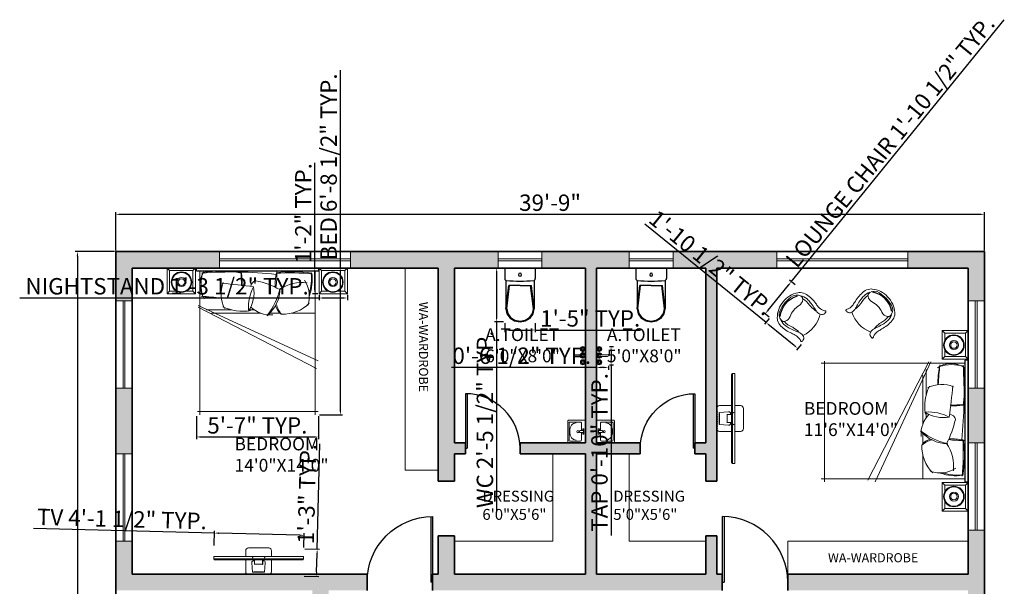
# Model space of a CAD drawing. Units: inches. Extents: x 4606 to 5879, y 1332 to 2209.
# Tile 4 of 7: x 4606 to 5147, y 1897 to 2209. Entities that reach past the tile are written whole.
import ezdxf

# ---------------------------------------------------------------- set-up
doc = ezdxf.new("R2010")
doc.units = ezdxf.units.IN
for name, color, linetype, lineweight in [('0.10', 252, 'Continuous', 9), ('0.15', 34, 'Continuous', 15), ('A-ANNO-DIMS', 2, 'Continuous', 18), ('A-ANNO-TEXT', 7, 'Continuous', 18), ('A-AREA-IDEN', 7, 'Continuous', 18), ('A-DOOR', 4, 'Continuous', 25), ('A-EQPM', 9, 'Continuous', 18), ('A-FLOR-CASE', 32, 'Continuous', 18), ('A-FURN', 8, 'Continuous', 18), ('A-WALL', 7, 'Continuous', 35), ('A-WALL-PATT', 252, 'Continuous', 13), ('window', 130, 'Continuous', 18), ('Сантехника', 9, 'Continuous', 18)]:
    doc.layers.add(name, color=color, linetype=linetype, lineweight=lineweight)
doc.layers.add('IFF-FURN-DETAIL', color=250, linetype='Continuous')
doc.layers.add('SANTEH', color=7, linetype='Continuous')
doc.styles.get("Standard").update_dxf_attribs({"font": 'arial.ttf'})
doc.dimstyles.new('ISO-25', dxfattribs={"dimtxt": 9, "dimasz": 2.5, "dimexe": 1.25, "dimexo": 0.625, "dimtad": 1, "dimlunit": 3, "dimtxsty": 'Standard', "dimcen": 2.5, "dimadec": 0, "dimazin": 0, "dimtfac": 1, "dimtmove": 0, "dimatfit": 3, "dimfxl": 1, "dimarcsym": 0})

# ---------------------------------------------------------------- blocks, each defined once
blk = doc.blocks.new('*D19')
at = {"layer": 'A-ANNO-DIMS', "color": 0, "lineweight": -2, "transparency": 16777216}
for p, q in [((4658.85, 2081.86), (4658.85, 2102.96)), ((4661.35, 2101.71), (5133.35, 2101.71)), ((5135.85, 2081.86), (5135.85, 2102.96))]:
    blk.add_line(p, q, dxfattribs=at)
at = {"layer": 'A-ANNO-DIMS', "color": 0, "transparency": 16777216}
for points in [[(4661.35, 2102.13), (4661.35, 2101.29), (4658.85, 2101.71)], [(5133.35, 2102.13), (5133.35, 2101.29), (5135.85, 2101.71)]]:
    blk.add_solid(points, dxfattribs=at)
at = {"layer": 'Defpoints', "color": 0, "transparency": 16777216}
for p in [(5135.85, 2101.71), (4658.85, 2081.24), (5135.85, 2081.24)]:
    blk.add_point(p, dxfattribs=at)
at = {"layer": 'A-ANNO-DIMS', "color": 0, "transparency": 16777216, "insert": (4897.35, 2106.93), "char_height": 9, "attachment_point": 5}
blk.add_mtext('39\'-9"', dxfattribs=at)
blk = doc.blocks.new('D1')
for p, q in [((0, 36), (0, 0)), ((1, 36), (1, 0)), ((0, 0), (1, 0))]:
    blk.add_line(p, q)
blk.add_arc((0, 0), 36, 0, 90)
blk = doc.blocks.new('D2')
for p, q in [((0, 30), (0, 0)), ((1, 30), (1, 0)), ((0, 0), (1, 0))]:
    blk.add_line(p, q)
blk.add_arc((0, 0), 30, 0, 90)
blk = doc.blocks.new('WC 2 Symb_109')
at = {"layer": 'SANTEH'}
for p, q in [((0, 0), (0, 380)), ((0, 380), (132, 380)), ((154, 365), (507, 365)), ((506, 365), (216, 331)), ((506, 356), (216, 322)), ((216, 190), (216, 331)), ((216, 190), (216, 49)), ((154, 15), (507, 15)), ((506, 24), (216, 58)), ((506, 15), (216, 49)), ((0, 0), (132, 0))]:
    blk.add_line(p, q, dxfattribs=at)
for points in [[(155, 360), (154, 364), (152, 368), (150, 371), (147, 374), (144, 377), (140, 379), (137, 380), (132, 380)], [(155, 20), (159, 62), (161, 105), (163, 147), (164, 190), (163, 233), (161, 275), (159, 318), (155, 360)], [(506, 24), (565, 37), (616, 73), (649, 126), (661, 190), (649, 254), (616, 307), (565, 343), (506, 356)], [(507, 15), (569, 28), (622, 66), (658, 123), (670, 190), (658, 257), (622, 314), (569, 352), (507, 365)], [(132, 0), (136, 0), (140, 1), (144, 3), (147, 6), (150, 9), (152, 12), (154, 16), (155, 20)]]:
    blk.add_lwpolyline(points, dxfattribs=at)
blk.add_lwpolyline([(84, 208), (70, 203), (65, 190), (70, 177), (84, 172), (97, 177), (102, 190), (97, 203)], close=True, dxfattribs=at)
blk = doc.blocks.new('Faucet - Bathroom top')
for p, q in [((-4.107, 0.125), (-4.375, 0.125)), ((-3.75, 0.4788), (-3.75, 0.75)), ((-3.5, 0.482), (-3.5, 0.75)), ((-3.1461, 0.125), (-2.875, 0.125)), ((3.143, 0.125), (2.875, 0.125)), ((3.5, 0.4788), (3.5, 0.75)), ((3.75, 0.482), (3.75, 0.75)), ((4.1039, 0.125), (4.375, 0.125)), ((-4.1039, -0.125), (-4.375, -0.125)), ((-3.75, -0.4821), (-3.75, -0.75)), ((-3.5, -0.4789), (-3.5, -0.75)), ((-3.143, -0.125), (-2.875, -0.125)), ((-0.5, -0.8639), (-0.5, -4.5)), ((0.5, -4.5), (0.5, -0.8631)), ((3.1461, -0.125), (2.875, -0.125)), ((3.5, -0.4821), (3.5, -0.75)), ((3.75, -0.4789), (3.75, -0.75)), ((4.107, -0.125), (4.375, -0.125))]:
    blk.add_line(p, q)
for centre, radius in [((-3.625, 0), 1.375), ((-4.625, 0), 0.2795), ((-3.625, 0), 0.5), ((-3.625, 1), 0.2795), ((-2.625, 0), 0.2795), ((0, 0), 0.5), ((3.625, 0), 1.375), ((2.625, 0), 0.2795), ((3.625, 0), 0.5), ((3.625, 1), 0.2795), ((4.625, 0), 0.2795), ((-3.625, -1), 0.2795), ((3.625, -1), 0.2795)]:
    blk.add_circle(centre, radius)
for centre, radius, start, end in [((-3.625, 0), 1, 105.2407, 164.2093), ((-3.625, 0), 1, 16.44125, 74.07887), ((0, 0), 1.5, 289.6514, 250.3603), ((0, 0), 1, 300.3431, 239.7554), ((3.625, 0), 1, 106.12, 164.0884), ((3.625, 0), 1, 16.23422, 73.90469), ((-3.625, 0), 1, 196.2342, 253.9047), ((-3.625, 0), 1, 286.12, 344.0884), ((0, -4.5), 0.5, 180, 0), ((3.625, 0), 1, 196.4413, 254.0789), ((3.625, 0), 1, 285.2407, 344.2093)]:
    blk.add_arc(centre, radius, start, end)
blk = doc.blocks.new('Rac7')
at = {"color": 0}
for p, q in [((-39501, -24232), (-39501, -23830)), ((-39474, -23808), (-38988, -23808)), ((-39457, -23859), (-39457, -24115)), ((-39032, -23838), (-39430, -23838)), ((-39221, -23855), (-39241, -23855)), ((-39005, -24115), (-39005, -23859)), ((-39005, -23859), (-39005, -23859)), ((-38961, -23830), (-38961, -24232)), ((-39253, -24186), (-39253, -24094)), ((-39209, -24186), (-39209, -24094)), ((-38961, -24232), (-39501, -24232)), ((-39430, -24136), (-39253, -24136)), ((-39297, -24164), (-39253, -24164)), ((-39297, -24194), (-39297, -24164)), ((-39165, -24194), (-39297, -24194)), ((-39253, -24186), (-39209, -24186)), ((-39209, -24136), (-39032, -24136)), ((-39209, -24164), (-39165, -24164)), ((-39165, -24164), (-39165, -24194))]:
    blk.add_line(p, q, dxfattribs=at)
at = {"color": 0, "extrusion": (0, 0, -1)}
for centre, major_axis, start_param, end_param in [((-39474, -23830), (-27, 0), 0, 1.570796), ((-39430, -23859), (-27, 0), 0, 1.570796), ((-39241, -24007), (-194, 0), 0, 1.570796), ((-39221, -24007), (-194, 0), 1.570796, 3.141593), ((-39032, -23859), (-27, 0), 1.570796, 3.141593), ((-38988, -23830), (-27, 0), 1.570796, 3.141593), ((-39231, -24104), (-25.3, 0), 0.552816, 2.588777), ((-39430, -24115), (-27, 0), -1.570796, 0), ((-39032, -24115), (-27, 0), -3.141593, -1.570796)]:
    blk.add_ellipse(centre, major_axis=major_axis, ratio=0.785714, start_param=start_param, end_param=end_param, dxfattribs=at)
blk.add_ellipse((-39231, -24048), major_axis=(-27.9, 0), ratio=0.785714, dxfattribs=at)
blk = doc.blocks.new('camita')
at = {"layer": '0.10'}
for p, q in [((-0.85, -0.045), (0.85, -0.045)), ((-0.805, -0.045), (-0.805, -2.048)), ((0.805, -0.045), (0.805, -2.048)), ((-0.827, -0.521), (0.846, -1.293)), ((-0.827, -0.548), (0.824, -1.399)), ((-0.716, -0.585), (-0.355, -0.585)), ((-0.638, -0.63), (0.043, -0.63)), ((-0.114, -0.585), (-0.049, -0.585)), ((0.175, -0.63), (0.318, -0.63)), ((0.474, -0.63), (0.805, -0.63)), ((-0.835, -2), (0.846, -2))]:
    blk.add_line(p, q, dxfattribs=at)
blk.add_lwpolyline([(-0.85, -0.041), (0.85, -0.041), (0.85, 0), (-0.85, 0)], close=True, dxfattribs=at)
for centre, radius, start, end in [((-0.457, -0.236), 0.344, 147.51, 213.8336), ((-0.2, -0.227), 0.586, 163.9263, 197.1409), ((-0.364, -5.846), 5.791, 83.8073, 94.1211), ((-0.51, -1.723), 1.678, 80.1255, 98.6619), ((2.353, -0.053), 2.58, 180.1063, 184.3854), ((-1.544, -0.245), 1.333, 359.9394, 7.5533), ((1.581, -0.289), 1.335, 170.3802, 178.9914), ((-1.44, -0.061), 1.712, 352.9291, 0.3959), ((0.452, -3.067), 3, 83.9026, 93.6759), ((0.486, -1.629), 1.578, 80.1602, 98.06), ((0.029, -0.138), 0.726, 342.5841, 6.0048), ((0.133, -0.17), 0.631, 339.923, 8.7433), ((-0.054, -0.363), 0.454, 159.3026, 206.5026), ((-1.33, -9.675), 9.499, 82.2708, 84.9399), ((0.458, -0.545), 0.584, 151.0456, 184.1497), ((-0.534, -0.339), 0.487, 327.2644, 9.0473), ((-0.007, -0.258), 0.0828, 100.018, 179.736), ((-0.293, -1.438), 1.29, 61.9749, 77.8435), ((0.627, -0.752), 0.551, 82.9691, 124.6739), ((0.32, -0.394), 0.404, 341.4524, 33.4512), ((-1.867, -14.986), 14.632, 84.6597, 85.7516), ((-0.46, 1.486), 1.909, 260.953, 268.6517), ((-0.199, -0.274), 0.516, 310.7395, 359.0576), ((-0.567, -0.087), 0.906, 321.6953, 346.4626), ((-0.2, 0.064), 0.667, 244.7809, 279.0606), ((0.179, -0.272), 0.383, 224.5284, 275.2229), ((0.438, -0.483), 0.19, 193.6849, 236.7035), ((0.571, -0.432), 0.315, 192.9388, 221.9636), ((0.361, -0.133), 0.51, 267.2589, 315.2997)]:
    blk.add_arc(centre, radius, start, end, dxfattribs=at)
blk = doc.blocks.new('VELADOR')
at = {"layer": '0.15'}
for p, q in [((-0.248, 0), (-0.203, -0.045)), ((0.248, 0), (0.202, -0.045)), ((-0.203, -0.405), (-0.248, -0.45)), ((0.248, -0.45), (0.202, -0.405))]:
    blk.add_line(p, q, dxfattribs=at)
blk.add_lwpolyline([(-0.248, 0), (-0.248, -0.45), (0.248, -0.45), (0.248, 0)], close=True, dxfattribs=at)
blk.add_lwpolyline([(0.092, -0.405), (0.202, -0.405), (0.202, -0.045), (-0.203, -0.045), (-0.203, -0.405), (-0.082, -0.405)], dxfattribs=at)
for radius in [0.18, 0.169, 0.0788, 0.0563]:
    blk.add_circle((0.005, -0.247), radius, dxfattribs=at)
blk = doc.blocks.new('TV')
at = {"color": 0}
for p, q in [((3967.27, 1784.85), (3967.05, 1784.65)), ((3967.76, 1763.68), (3967.54, 1763.86))]:
    blk.add_line(p, q, dxfattribs=at)
at = {"layer": 'window'}
for p, q in [((3967.54, 1763.86), (3967.05, 1784.65)), ((3964.41, 1777.23), (3967.22, 1777.3)), ((3968.01, 1777.32), (3969.36, 1777.35)), ((3966.53, 1775.82), (3964.33, 1775.61)), ((3964.34, 1775.34), (3964.45, 1775.34)), ((3964.34, 1775.31), (3964.43, 1775.32)), ((3966.14, 1775.2), (3967.01, 1775.22)), ((3966.14, 1775.18), (3967.27, 1775.2)), ((3966.14, 1775.18), (3966.14, 1775.2)), ((3966.3, 1773.29), (3966.26, 1775.18)), ((3964.39, 1773.06), (3964.48, 1773.06)), ((3964.39, 1773.04), (3964.5, 1773.04)), ((3966.61, 1772.66), (3964.4, 1772.77)), ((3966.19, 1773.28), (3967.31, 1773.31)), ((3966.19, 1773.26), (3967.05, 1773.28)), ((3966.19, 1773.26), (3966.19, 1773.28)), ((3964.55, 1771.15), (3967.36, 1771.22)), ((3968.15, 1771.24), (3969.5, 1771.27))]:
    blk.add_line(p, q, dxfattribs=at)
for points in [[(3968.33, 1763.69), (3967.83, 1784.86), (3967.27, 1784.85), (3967.76, 1763.68), (3968.33, 1763.69)], [(3963.86, 1771.81), (3963.75, 1776.54)], [(3964.4, 1772.77), (3964.33, 1775.61)], [(3964.48, 1773.06), (3964.43, 1775.32)], [(3964.5, 1773.04), (3964.45, 1775.34)], [(3970.16, 1771.96), (3970.05, 1776.69)]]:
    blk.add_lwpolyline(points, dxfattribs=at)
for points in [[(3966.53, 1775.82, -0.263666), (3966.93, 1775.69), (3967, 1775.57), (3967.01, 1775.22)], [(3966.61, 1772.66, 0.263666), (3967, 1772.81), (3967.06, 1772.93), (3967.05, 1773.28)]]:
    blk.add_lwpolyline(points, format="xyb", dxfattribs=at)
for centre, radius in [((3963.91, 1775.73), 0.0679), ((3963.93, 1775.17), 0.0679), ((3967.77, 1775.68), 0.0451), ((3963.94, 1774.6), 0.0679), ((3963.95, 1774.04), 0.0679), ((3963.97, 1773.48), 0.0679), ((3963.98, 1772.92), 0.0679), ((3967.83, 1772.86), 0.0451), ((3963.99, 1772.35), 0.0679), ((3964.01, 1771.79), 0.0679)]:
    blk.add_circle(centre, radius, dxfattribs=at)
for centre, start, end in [((3964.42, 1776.56), 91.3414, 181.3414), ((3969.38, 1776.67), 1.3414, 91.3414), ((3964.53, 1771.83), 181.3414, 271.3414), ((3969.49, 1771.94), 271.3414, 1.3414)]:
    blk.add_arc(centre, 0.676, start, end, dxfattribs=at)
blk = doc.blocks.new('ILNG95')
for points in [[(120, 308, -0.32971), (51, 384, -0.036099), (50, 422, -0.497733), (75, 439, -0.070621), (96, 429, 0.101868), (133, 414, 0.091794), (259, 412, 0.024114), (351, 433, -0.090294), (638, 458, -0.132412), (775, 407, -0.068618), (816, 368, -0.184346), (943, 0, 1.803905)], [(120, 308, 0.138132), (244, 313, 0.001085), (325, 339, -0.034227), (462, 375, -0.033255), (567, 387, -0.137428), (727, 350, -4.561553)], [(120, 308, 0.138132), (244, 313, 0.001085), (325, 339, -0.034227), (462, 375, -0.033255), (567, 387, -0.137428), (727, 350, -4.561553)], [(235, 308, 0.064243), (394, 307, 0.04414), (433, 315, -0.118032), (643, 329, -6.296816)], [(235, 308, 0.064243), (394, 307, 0.04414), (433, 315, -0.118032), (643, 329, -6.296816)], [(639, 0, 0.078302), (612, 161, -0.233633), (633, 315, -0.28763), (710, 349, -0.317923), (875, 193, -0.032882), (900, 0, 1.140397)], [(639, 0, 0.078302), (612, 161, -0.233633), (633, 315, -0.28763), (710, 349, -0.317923), (875, 193, -0.032882), (900, 0, 1.140397)], [(120, -308, 0.32971), (51, -384, 0.036099), (50, -422, 0.497733), (75, -439, 0.070621), (96, -429, -0.101868), (133, -414, -0.091794), (259, -412, -0.024114), (351, -433, 0.090294), (638, -458, 0.132412), (775, -407, 0.068618), (816, -368, 0.184346), (943, 0, -1.803905)], [(639, 0, -0.078302), (612, -161, 0.233633), (633, -315, 0.28763), (710, -349, 0.317923), (875, -193, 0.032882), (900, 0, -1.140397)], [(639, 0, -0.078302), (612, -161, 0.233633), (633, -315, 0.28763), (710, -349, 0.317923), (875, -193, 0.032882), (900, 0, -1.140397)], [(120, -308, -0.138132), (244, -313, -0.001085), (325, -339, 0.034227), (462, -375, 0.033255), (567, -387, 0.137428), (727, -350, 4.561553)], [(120, -308, -0.138132), (244, -313, -0.001085), (325, -339, 0.034227), (462, -375, 0.033255), (567, -387, 0.137428), (727, -350, 4.561553)], [(235, -308, -0.064243), (394, -307, -0.04414), (433, -315, 0.118032), (643, -329, 6.296816)], [(235, -308, -0.064243), (394, -307, -0.04414), (433, -315, 0.118032), (643, -329, 6.296816)]]:
    blk.add_lwpolyline(points, format="xyb")
blk.add_arc((759, 1), 709, 154.3281, 205.801)
at = {"layer": 'IFF-FURN-DETAIL'}
blk.add_arc((326, -2), 549, 326.8997, 34.6691, dxfattribs=at)
blk.add_arc((326, -2), 549, 326.8997, 34.6691, dxfattribs=at)
blk = doc.blocks.new('*D24')
at = {"layer": 'A-ANNO-DIMS', "color": 0, "lineweight": -2, "transparency": 16777216}
for p, q in [((4658.23, 2081.24), (4636.6, 2081.24)), ((4637.85, 2078.74), (4637.85, 1413.74)), ((4658.23, 1411.24), (4636.6, 1411.24))]:
    blk.add_line(p, q, dxfattribs=at)
at = {"layer": 'A-ANNO-DIMS', "color": 0, "transparency": 16777216}
for points in [[(4637.43, 2078.74), (4638.26, 2078.74), (4637.85, 2081.24)], [(4637.43, 1413.74), (4638.26, 1413.74), (4637.85, 1411.24)]]:
    blk.add_solid(points, dxfattribs=at)
at = {"layer": 'Defpoints', "color": 0, "transparency": 16777216}
for p in [(4658.85, 2081.24), (4637.85, 1411.24), (4658.85, 1411.24)]:
    blk.add_point(p, dxfattribs=at)
at = {"layer": 'A-ANNO-DIMS', "color": 0, "transparency": 16777216, "insert": (4632.62, 1746.24), "char_height": 9, "attachment_point": 5, "rotation": 90}
blk.add_mtext('55\'-10"', dxfattribs=at)
blk = doc.blocks.new('GLAZING-72IN')
for p, q in [((0, 0), (0, 72)), ((1, 0), (1, 72))]:
    blk.add_line(p, q)
blk = doc.blocks.new('GLAZING-24IN')
for p, q in [((0, 0), (0, 24)), ((1, 0), (1, 24))]:
    blk.add_line(p, q)
blk = doc.blocks.new('GLAZING-48IN')
for p, q in [((0, 0), (0, 48)), ((1, 0), (1, 48))]:
    blk.add_line(p, q)
blk = doc.blocks.new('*D89')
at = {"layer": 'A-ANNO-DIMS', "color": 0, "lineweight": -2, "transparency": 16777216}
for p, q in [((4770.49, 2055.77), (4606.12, 2055.77)), ((4770.49, 2057.48), (4770.49, 2054.52)), ((4783.54, 2055.77), (4772.99, 2055.77)), ((4786.04, 2057.48), (4786.04, 2054.52))]:
    blk.add_line(p, q, dxfattribs=at)
at = {"layer": 'A-ANNO-DIMS', "color": 0, "transparency": 16777216}
for points in [[(4772.99, 2056.19), (4772.99, 2055.35), (4770.49, 2055.77)], [(4783.54, 2056.19), (4783.54, 2055.35), (4786.04, 2055.77)]]:
    blk.add_solid(points, dxfattribs=at)
at = {"layer": 'Defpoints', "color": 0, "transparency": 16777216}
for p in [(4770.49, 2058.1), (4770.49, 2055.77), (4786.04, 2058.1)]:
    blk.add_point(p, dxfattribs=at)
at = {"layer": 'A-ANNO-DIMS', "color": 0, "transparency": 16777216, "insert": (4687.05, 2061.05), "char_height": 9, "attachment_point": 5}
blk.add_mtext('NIGHTSTAND 1\'-3 1/2" TYP.', dxfattribs=at)
blk = doc.blocks.new('*D90')
at = {"layer": 'A-ANNO-DIMS', "color": 0, "lineweight": -2, "transparency": 16777216}
for p, q in [((4768.15, 2072.24), (4768.15, 2130)), ((4769.86, 2072.24), (4766.9, 2072.24)), ((4768.15, 2060.6), (4768.15, 2069.74)), ((4769.86, 2058.1), (4766.9, 2058.1))]:
    blk.add_line(p, q, dxfattribs=at)
at = {"layer": 'A-ANNO-DIMS', "color": 0, "transparency": 16777216}
for points in [[(4767.74, 2069.74), (4768.57, 2069.74), (4768.15, 2072.24)], [(4767.74, 2060.6), (4768.57, 2060.6), (4768.15, 2058.1)]]:
    blk.add_solid(points, dxfattribs=at)
at = {"layer": 'Defpoints', "color": 0, "transparency": 16777216}
for p in [(4768.15, 2072.24), (4770.49, 2072.24), (4770.49, 2058.1)]:
    blk.add_point(p, dxfattribs=at)
at = {"layer": 'A-ANNO-DIMS', "color": 0, "transparency": 16777216, "insert": (4763.01, 2102.37), "char_height": 9, "attachment_point": 5, "rotation": 90}
blk.add_mtext('1\'-2" TYP.', dxfattribs=at)
blk = doc.blocks.new('*D91')
at = {"layer": 'A-ANNO-DIMS', "color": 0, "lineweight": -2, "transparency": 16777216}
for p, q in [((4871.83, 2072.24), (4866.76, 2072.24)), ((4868.01, 2069.74), (4868.01, 2045.13)), ((4871.83, 2042.63), (4866.76, 2042.63)), ((4868.01, 2042.63), (4868.01, 1938.24))]:
    blk.add_line(p, q, dxfattribs=at)
at = {"layer": 'A-ANNO-DIMS', "color": 0, "transparency": 16777216}
for points in [[(4867.6, 2069.74), (4868.43, 2069.74), (4868.01, 2072.24)], [(4867.6, 2045.13), (4868.43, 2045.13), (4868.01, 2042.63)]]:
    blk.add_solid(points, dxfattribs=at)
at = {"layer": 'Defpoints', "color": 0, "transparency": 16777216}
for p in [(4872.45, 2072.24), (4868.01, 2042.63), (4872.45, 2042.63)]:
    blk.add_point(p, dxfattribs=at)
at = {"layer": 'A-ANNO-DIMS', "color": 0, "transparency": 16777216, "insert": (4862.73, 1989.19), "char_height": 9, "attachment_point": 5, "rotation": 90}
blk.add_mtext('WC 2\'-5 1/2" TYP.', dxfattribs=at)
blk = doc.blocks.new('*D92')
at = {"layer": 'A-ANNO-DIMS', "color": 0, "lineweight": -2, "transparency": 16777216}
for p, q in [((4872.45, 2042.01), (4872.45, 2036.94)), ((4889.25, 2042.01), (4889.25, 2036.94)), ((4874.95, 2038.19), (4886.75, 2038.19)), ((4889.25, 2038.19), (4947.01, 2038.19))]:
    blk.add_line(p, q, dxfattribs=at)
at = {"layer": 'A-ANNO-DIMS', "color": 0, "transparency": 16777216}
for points in [[(4874.95, 2038.61), (4874.95, 2037.77), (4872.45, 2038.19)], [(4886.75, 2038.61), (4886.75, 2037.77), (4889.25, 2038.19)]]:
    blk.add_solid(points, dxfattribs=at)
at = {"layer": 'Defpoints', "color": 0, "transparency": 16777216}
for p in [(4872.45, 2042.63), (4889.25, 2042.63), (4889.25, 2038.19)]:
    blk.add_point(p, dxfattribs=at)
at = {"layer": 'A-ANNO-DIMS', "color": 0, "transparency": 16777216, "insert": (4919.38, 2043.41), "char_height": 9, "attachment_point": 5}
blk.add_mtext('1\'-5" TYP.', dxfattribs=at)
blk = doc.blocks.new('*D93')
at = {"layer": 'A-ANNO-DIMS', "color": 0, "lineweight": -2, "transparency": 16777216}
for p, q in [((4929.98, 2029.13), (4932.1, 2029.13)), ((4930.85, 2026.63), (4930.85, 2021.63)), ((4929.98, 2019.13), (4932.1, 2019.13)), ((4930.85, 2019.13), (4930.85, 1925.36))]:
    blk.add_line(p, q, dxfattribs=at)
at = {"layer": 'A-ANNO-DIMS', "color": 0, "transparency": 16777216}
for points in [[(4930.43, 2026.63), (4931.27, 2026.63), (4930.85, 2029.13)], [(4930.43, 2021.63), (4931.27, 2021.63), (4930.85, 2019.13)]]:
    blk.add_solid(points, dxfattribs=at)
at = {"layer": 'Defpoints', "color": 0, "transparency": 16777216}
for p in [(4929.35, 2029.13), (4929.35, 2019.13), (4930.85, 2019.13)]:
    blk.add_point(p, dxfattribs=at)
at = {"layer": 'A-ANNO-DIMS', "color": 0, "transparency": 16777216, "insert": (4925.63, 1971), "char_height": 9, "attachment_point": 5, "rotation": 90}
blk.add_mtext('TAP 0\'-10" TYP.', dxfattribs=at)
blk = doc.blocks.new('*D94')
at = {"layer": 'A-ANNO-DIMS', "color": 0, "lineweight": -2, "transparency": 16777216}
for p, q in [((4922.85, 2017.63), (4843.27, 2017.63)), ((4922.85, 2018.51), (4922.85, 2016.38)), ((4926.85, 2017.63), (4925.35, 2017.63)), ((4929.35, 2018.51), (4929.35, 2016.38))]:
    blk.add_line(p, q, dxfattribs=at)
at = {"layer": 'A-ANNO-DIMS', "color": 0, "transparency": 16777216}
for points in [[(4925.35, 2018.05), (4925.35, 2017.22), (4922.85, 2017.63)], [(4926.85, 2018.05), (4926.85, 2017.22), (4929.35, 2017.63)]]:
    blk.add_solid(points, dxfattribs=at)
at = {"layer": 'Defpoints', "color": 0, "transparency": 16777216}
for p in [(4922.85, 2019.13), (4922.85, 2017.63), (4929.35, 2019.13)]:
    blk.add_point(p, dxfattribs=at)
at = {"layer": 'A-ANNO-DIMS', "color": 0, "transparency": 16777216, "insert": (4881.81, 2022.91), "char_height": 9, "attachment_point": 5}
blk.add_mtext('0\'-6 1/2" TYP.', dxfattribs=at)
blk = doc.blocks.new('*D95')
at = {"layer": 'A-ANNO-DIMS', "color": 0, "lineweight": -2, "transparency": 16777216}
for p, q in [((4782.21, 2072.24), (4782.21, 2180.77)), ((4770.74, 2072.24), (4783.46, 2072.24)), ((4782.21, 1994.08), (4782.21, 2069.74)), ((4770.74, 1991.58), (4783.46, 1991.58))]:
    blk.add_line(p, q, dxfattribs=at)
at = {"layer": 'A-ANNO-DIMS', "color": 0, "transparency": 16777216}
for points in [[(4781.79, 2069.74), (4782.63, 2069.74), (4782.21, 2072.24)], [(4781.79, 1994.08), (4782.63, 1994.08), (4782.21, 1991.58)]]:
    blk.add_solid(points, dxfattribs=at)
at = {"layer": 'Defpoints', "color": 0, "transparency": 16777216}
for p in [(4770.11, 2072.24), (4782.21, 2072.24), (4770.11, 1991.58)]:
    blk.add_point(p, dxfattribs=at)
at = {"layer": 'A-ANNO-DIMS', "color": 0, "transparency": 16777216, "insert": (4776.93, 2127.75), "char_height": 9, "attachment_point": 5, "rotation": 90}
blk.add_mtext('BED 6\'-8 1/2" TYP.', dxfattribs=at)
blk = doc.blocks.new('*D96')
at = {"layer": 'A-ANNO-DIMS', "color": 0, "lineweight": -2, "transparency": 16777216}
for p, q in [((4703.17, 1990.96), (4703.17, 1978.23)), ((4770.11, 1990.96), (4770.11, 1978.23)), ((4705.67, 1979.48), (4767.61, 1979.48))]:
    blk.add_line(p, q, dxfattribs=at)
at = {"layer": 'A-ANNO-DIMS', "color": 0, "transparency": 16777216}
for points in [[(4705.67, 1979.9), (4705.67, 1979.07), (4703.17, 1979.48)], [(4767.61, 1979.9), (4767.61, 1979.07), (4770.11, 1979.48)]]:
    blk.add_solid(points, dxfattribs=at)
at = {"layer": 'Defpoints', "color": 0, "transparency": 16777216}
for p in [(4703.17, 1991.58), (4770.11, 1991.58), (4770.11, 1979.48)]:
    blk.add_point(p, dxfattribs=at)
at = {"layer": 'A-ANNO-DIMS', "color": 0, "transparency": 16777216, "insert": (4736.64, 1984.68), "char_height": 9, "attachment_point": 5}
blk.add_mtext('5\'-7" TYP.', dxfattribs=at)
blk = doc.blocks.new('*D97')
at = {"layer": 'A-ANNO-DIMS', "color": 0, "lineweight": -2, "transparency": 16777216}
for p, q in [((4713, 1926.73), (4613.66, 1929.26)), ((4712.83, 1919.96), (4713.03, 1927.98)), ((4759.79, 1925.54), (4715.5, 1926.67)), ((4762.11, 1918.71), (4762.32, 1926.72))]:
    blk.add_line(p, q, dxfattribs=at)
at = {"layer": 'A-ANNO-DIMS', "color": 0, "transparency": 16777216}
for points in [[(4715.51, 1927.08), (4715.49, 1926.25), (4713, 1926.73)], [(4759.8, 1925.96), (4759.78, 1925.12), (4762.29, 1925.48)]]:
    blk.add_solid(points, dxfattribs=at)
at = {"layer": 'Defpoints', "color": 0, "transparency": 16777216}
for p in [(4713, 1926.73), (4712.81, 1919.34), (4762.1, 1918.08)]:
    blk.add_point(p, dxfattribs=at)
at = {"layer": 'A-ANNO-DIMS', "color": 0, "transparency": 16777216, "insert": (4662.21, 1933.3), "char_height": 9, "attachment_point": 5, "rotation": 358.5431}
blk.add_mtext('TV 4\'-1 1/2" TYP.', dxfattribs=at)
blk = doc.blocks.new('*D98')
at = {"layer": 'A-ANNO-DIMS', "color": 0, "lineweight": -2, "transparency": 16777216}
for p, q in [((4769.49, 1917.89), (4770.96, 1975.64)), ((4762.72, 1918.07), (4770.74, 1917.86)), ((4769.17, 1905.44), (4769.43, 1915.39)), ((4762.34, 1903.12), (4770.36, 1902.91))]:
    blk.add_line(p, q, dxfattribs=at)
at = {"layer": 'A-ANNO-DIMS', "color": 0, "transparency": 16777216}
for points in [[(4769.01, 1915.41), (4769.84, 1915.38), (4769.49, 1917.89)], [(4768.76, 1905.45), (4769.59, 1905.43), (4769.11, 1902.94)]]:
    blk.add_solid(points, dxfattribs=at)
at = {"layer": 'Defpoints', "color": 0, "transparency": 16777216}
for p in [(4762.1, 1918.08), (4769.49, 1917.89), (4761.72, 1903.13)]:
    blk.add_point(p, dxfattribs=at)
at = {"layer": 'A-ANNO-DIMS', "color": 0, "transparency": 16777216, "insert": (4765.03, 1948.15), "char_height": 9, "attachment_point": 5, "rotation": 88.5431}
blk.add_mtext('1\'-3" TYP.', dxfattribs=at)
blk = doc.blocks.new('*D99')
at = {"layer": 'A-ANNO-DIMS', "color": 0, "lineweight": -2, "transparency": 16777216}
for p, q in [((5029.81, 2064.74), (5146.76, 2208.57)), ((5031.97, 2062.98), (5028.84, 2065.53)), ((5017.04, 2049.03), (5028.23, 2062.8)), ((5017.62, 2045.33), (5014.49, 2047.88))]:
    blk.add_line(p, q, dxfattribs=at)
at = {"layer": 'A-ANNO-DIMS', "color": 0, "transparency": 16777216}
for points in [[(5027.91, 2063.06), (5028.56, 2062.53), (5029.81, 2064.74)], [(5016.72, 2049.29), (5017.36, 2048.76), (5015.46, 2047.09)]]:
    blk.add_solid(points, dxfattribs=at)
at = {"layer": 'Defpoints', "color": 0, "transparency": 16777216}
for p in [(5029.81, 2064.74), (5032.46, 2062.58), (5018.11, 2044.93)]:
    blk.add_point(p, dxfattribs=at)
at = {"layer": 'A-ANNO-DIMS', "color": 0, "transparency": 16777216, "insert": (5084.98, 2140.95), "char_height": 9, "attachment_point": 5, "rotation": 50.8857}
blk.add_mtext('LOUNGE CHAIR 1\'-10 1/2" TYP.', dxfattribs=at)
blk = doc.blocks.new('*D100')
at = {"layer": 'A-ANNO-DIMS', "color": 0, "lineweight": -2, "transparency": 16777216}
for p, q in [((5015.96, 2042.29), (4949.44, 2096.37)), ((5017.71, 2044.45), (5015.17, 2041.32)), ((5031.43, 2029.71), (5017.9, 2040.71)), ((5035.13, 2030.29), (5032.58, 2027.16))]:
    blk.add_line(p, q, dxfattribs=at)
at = {"layer": 'A-ANNO-DIMS', "color": 0, "transparency": 16777216}
for points in [[(5018.16, 2041.03), (5017.63, 2040.39), (5015.96, 2042.29)], [(5031.69, 2030.03), (5031.17, 2029.38), (5033.37, 2028.13)]]:
    blk.add_solid(points, dxfattribs=at)
at = {"layer": 'Defpoints', "color": 0, "transparency": 16777216}
for p in [(5018.11, 2044.93), (5015.96, 2042.29), (5035.52, 2030.78)]:
    blk.add_point(p, dxfattribs=at)
at = {"layer": 'A-ANNO-DIMS', "color": 0, "transparency": 16777216, "insert": (4985.06, 2074.21), "char_height": 9, "attachment_point": 5, "rotation": 320.8857}
blk.add_mtext('1\'-10 1/2" TYP.', dxfattribs=at)

msp = doc.modelspace()

# ---------------------------------------------------------------- hatches: boundary and pattern name
at = {"layer": 'A-WALL-PATT', "transparency": 33554687}
h = msp.add_hatch(color=256, dxfattribs=at)
h.dxf.hatch_style = 1
h.paths.add_polyline_path([(4715.85, 2081.239), (4658.85, 2081.239), (4658.85, 2054.239), (4667.85, 2054.239), (4667.85, 2072.239), (4715.85, 2072.239)])
h.paths.add_polyline_path([(4868.85, 2081.239), (4787.85, 2081.239), (4787.85, 2072.239), (4835.85, 2072.239), (4835.85, 1955.239), (4844.85, 1955.239), (4844.85, 1970.239), (4850.85, 1970.239), (4850.85, 1976.239), (4844.85, 1976.239), (4844.85, 2072.239), (4868.85, 2072.239)])
h.paths.add_polyline_path([(4940.85, 2081.239), (4892.85, 2081.239), (4892.85, 2072.239), (4916.85, 2072.239), (4916.85, 1976.239), (4880.85, 1976.239), (4880.85, 1970.239), (4916.85, 1970.239), (4916.85, 1904.239), (4844.85, 1904.239), (4844.85, 1925.239), (4835.85, 1925.239), (4835.85, 1904.239), (4832.85, 1904.239), (4832.85, 1895.239), (4919.85, 1895.239), (4991.85, 1895.239), (4991.85, 1904.239), (4988.85, 1904.239), (4988.85, 1925.239), (4982.85, 1925.239), (4982.85, 1904.239), (4922.85, 1904.239), (4922.85, 1970.239), (4946.85, 1970.239), (4946.85, 1976.239), (4922.85, 1976.239), (4922.85, 2072.239), (4940.85, 2072.239)])
h.paths.add_polyline_path([(5021.85, 2081.239), (4964.85, 2081.239), (4964.85, 2072.239), (4982.85, 2072.239), (4982.85, 1976.239), (4976.85, 1976.239), (4976.85, 1970.239), (4982.85, 1970.239), (4982.85, 1955.239), (4988.85, 1955.239), (4988.85, 2072.239), (5021.85, 2072.239)])
h.paths.add_polyline_path([(5135.85, 2081.239), (5093.85, 2081.239), (5093.85, 2072.239), (5126.85, 2072.239), (5126.85, 2054.239), (5135.85, 2054.239)])
h.paths.add_polyline_path([(5135.85, 2006.239), (5126.85, 2006.239), (5126.85, 1976.239), (5135.85, 1976.239)])
h.paths.add_polyline_path([(5135.85, 1928.239), (5126.85, 1928.239), (5126.85, 1904.239), (5027.85, 1904.239), (5027.85, 1895.239), (5126.85, 1895.239), (5126.85, 1871.239), (5135.85, 1871.239)])
h.paths.add_polyline_path([(4796.85, 1904.239), (4667.85, 1904.239), (4667.85, 1922.239), (4658.85, 1922.239), (4658.85, 1895.239), (4766.85, 1895.239), (4766.85, 1674.239), (4775.85, 1674.239), (4775.85, 1895.239), (4796.85, 1895.239)])
h.paths.add_polyline_path([(4667.85, 2006.239), (4658.85, 2006.239), (4658.85, 1970.239), (4667.85, 1970.239)])
h.paths.add_polyline_path([(4880.85, 1545.239), (4940.85, 1545.239), (4940.85, 1542.239), (4949.85, 1542.239), (4949.85, 1566.239), (4940.85, 1566.239), (4940.85, 1554.239), (4880.85, 1554.239), (4880.85, 1614.239), (4940.85, 1614.239), (4940.85, 1602.239), (4949.85, 1602.239), (4949.85, 1623.239), (4866.739, 1623.239), (4826.85, 1623.239), (4826.85, 1614.239), (4871.85, 1614.239), (4871.85, 1554.239), (4826.85, 1554.239), (4826.85, 1545.239), (4871.85, 1545.239), (4871.85, 1411.239), (4997.85, 1411.239), (4997.85, 1420.239), (4949.85, 1420.239), (4949.85, 1512.239), (4940.85, 1512.239), (4940.85, 1420.239), (4880.85, 1420.239)])
h.paths.add_polyline_path([(5102.85, 1446.239), (5093.85, 1446.239), (5093.85, 1420.239), (5045.85, 1420.239), (5045.85, 1411.239), (5102.85, 1411.239)])
h.paths.add_polyline_path([(5102.85, 1591.739), (5093.85, 1591.739), (5093.85, 1542.239), (5102.85, 1542.239)])
h.paths.add_polyline_path([(5135.85, 1691.239), (5126.85, 1691.239), (5126.85, 1673.239), (5030.85, 1673.239), (5030.85, 1676.239), (5021.85, 1676.239), (5021.85, 1673.239), (5003.85, 1673.239), (5003.85, 1664.239), (5093.85, 1664.239), (5093.85, 1639.739), (5102.85, 1639.739), (5102.85, 1664.239), (5135.85, 1664.239)])
h.paths.add_polyline_path([(5135.85, 1823.239), (5126.85, 1823.239), (5126.85, 1799.239), (5028.85, 1799.239), (5028.85, 1790.239), (5057.85, 1790.239), (5057.85, 1784.239), (5066.85, 1784.239), (5066.85, 1790.239), (5126.85, 1790.239), (5126.85, 1742.239), (5066.85, 1742.239), (5066.85, 1748.239), (5057.85, 1748.239), (5057.85, 1742.239), (5021.85, 1742.239), (5021.85, 1706.239), (5030.85, 1706.239), (5030.85, 1733.239), (5126.85, 1733.239), (5126.85, 1715.239), (5135.85, 1715.239)])
h.paths.add_polyline_path([(4775.85, 1602.239), (4766.85, 1602.239), (4766.85, 1474.239), (4775.85, 1474.239), (4775.85, 1545.239), (4778.85, 1545.239), (4778.85, 1554.239), (4775.85, 1554.239)])
h.paths.add_polyline_path([(4692.58, 1635.003), (4749.356, 1635.003), (4749.356, 1665.418), (4692.58, 1665.418)], flags=9)

# ---------------------------------------------------------------- linework, layer by layer
at = {"layer": 'A-FLOR-CASE'}
for p, q in [((4817.85, 2072.239), (4817.85, 1961.239)), ((4898.85, 1970.239), (4898.85, 1922.239)), ((4940.85, 1970.239), (4940.85, 1922.239)), ((4817.85, 1961.239), (4835.85, 1961.239)), ((4898.85, 1922.239), (4844.85, 1922.239)), ((4982.85, 1922.239), (4940.85, 1922.239)), ((5126.85, 1922.239), (5027.85, 1922.239)), ((5027.85, 1904.239), (5027.85, 1922.239))]:
    msp.add_line(p, q, dxfattribs=at)
at = {"layer": 'A-WALL'}
for p, q in [((4667.85, 2072.239), (4667.85, 1904.239)), ((4835.85, 2072.239), (4667.85, 2072.239)), ((4835.85, 2072.239), (4835.85, 1955.239)), ((4844.85, 2072.239), (4844.85, 1976.239)), ((4916.85, 2072.239), (4844.85, 2072.239)), ((4916.85, 2072.239), (4916.85, 1976.239)), ((4922.85, 2072.239), (4922.85, 1976.239)), ((4982.85, 2072.239), (4922.85, 2072.239)), ((4982.85, 2072.239), (4982.85, 1976.239)), ((5126.85, 2072.239), (4988.85, 2072.239)), ((4988.85, 2072.239), (4988.85, 1955.239)), ((5126.85, 1904.239), (5126.85, 2072.239)), ((4850.85, 1976.239), (4844.85, 1976.239)), ((4850.85, 1976.239), (4850.85, 1970.239)), ((4916.85, 1976.239), (4880.85, 1976.239)), ((4880.85, 1976.239), (4880.85, 1970.239)), ((4946.85, 1976.239), (4922.85, 1976.239)), ((4946.85, 1976.239), (4946.85, 1970.239)), ((4982.85, 1976.239), (4976.85, 1976.239)), ((4976.85, 1976.239), (4976.85, 1970.239)), ((4844.85, 1970.239), (4844.85, 1955.239)), ((4850.85, 1970.239), (4844.85, 1970.239)), ((4916.85, 1970.239), (4880.85, 1970.239)), ((4916.85, 1970.239), (4916.85, 1904.239)), ((4922.85, 1970.239), (4922.85, 1904.239)), ((4946.85, 1970.239), (4922.85, 1970.239)), ((4982.85, 1970.239), (4976.85, 1970.239)), ((4982.85, 1970.239), (4982.85, 1955.239)), ((4844.85, 1955.239), (4835.85, 1955.239)), ((4988.85, 1955.239), (4982.85, 1955.239)), ((4835.85, 1925.239), (4835.85, 1904.239)), ((4844.85, 1925.239), (4835.85, 1925.239)), ((4844.85, 1925.239), (4844.85, 1904.239)), ((4988.85, 1925.239), (4982.85, 1925.239)), ((4982.85, 1925.239), (4982.85, 1904.239)), ((4988.85, 1925.239), (4988.85, 1904.239)), ((4796.85, 1904.239), (4667.85, 1904.239)), ((4796.85, 1904.239), (4796.85, 1895.239)), ((4835.85, 1904.239), (4832.85, 1904.239)), ((4832.85, 1904.239), (4832.85, 1895.239)), ((4916.85, 1904.239), (4844.85, 1904.239)), ((4982.85, 1904.239), (4922.85, 1904.239)), ((4991.85, 1904.239), (4988.85, 1904.239)), ((4991.85, 1904.239), (4991.85, 1895.239)), ((5126.85, 1904.239), (5027.85, 1904.239)), ((5027.85, 1904.239), (5027.85, 1895.239))]:
    msp.add_line(p, q, dxfattribs=at)
msp.add_lwpolyline([(5135.85, 1664.239), (5135.85, 2081.239), (4658.85, 2081.239), (4658.85, 1411.239), (5102.85, 1411.239)], dxfattribs=at)
at = {"layer": 'window'}
for p, q in [((4715.85, 2072.239), (4715.85, 2081.239)), ((4787.85, 2072.239), (4787.85, 2081.239)), ((4868.85, 2072.239), (4868.85, 2081.239)), ((4892.85, 2072.239), (4892.85, 2081.239)), ((4940.85, 2072.239), (4940.85, 2081.239)), ((4964.85, 2072.239), (4964.85, 2081.239)), ((5021.85, 2072.239), (5021.85, 2081.239)), ((5093.85, 2072.239), (5093.85, 2081.239)), ((4667.85, 2054.239), (4658.85, 2054.239)), ((5135.85, 2054.239), (5126.85, 2054.239)), ((4667.85, 2006.239), (4658.85, 2006.239)), ((5135.85, 2006.239), (5126.85, 2006.239)), ((5135.85, 1976.239), (5126.85, 1976.239)), ((4667.85, 1970.239), (4658.85, 1970.239)), ((5135.85, 1928.239), (5126.85, 1928.239)), ((4667.85, 1922.239), (4658.85, 1922.239))]:
    msp.add_line(p, q, dxfattribs=at)

# ---------------------------------------------------------------- block references
at = {"layer": 'A-DOOR'}
for name, p in [('D2', (4850.85, 1973.239)), ('D1', (4991.85, 1899.739))]:
    msp.add_blockref(name, p, dxfattribs=at)
at = {"layer": 'A-DOOR', "xscale": -1}
for name, p in [('D2', (4976.85, 1973.239)), ('D1', (4832.85, 1899.739))]:
    msp.add_blockref(name, p, dxfattribs=at)
at = {"layer": 'A-EQPM', "xscale": 2.327319231123021, "yscale": 2.327319231123021, "zscale": 2.327319231123021}
for p, rotation in [((-4338.179, -1903.573), 358.5430845181613), ((8630.484, -7423.138), 88.54308451816127)]:
    msp.add_blockref('TV', p, dxfattribs=dict(at, rotation=rotation))
at = {"layer": 'A-FURN'}
for name, p, xscale, yscale, zscale in [('VELADOR', (4694.812, 2072.239), 31.41542173157097, 31.41542173157097, 31.41542173157097), ('camita', (4736.643, 2072.239), 39.375, 39.375, 39.375)]:
    msp.add_blockref(name, p, dxfattribs=dict(at, xscale=xscale, yscale=yscale, zscale=zscale))
for name, p, xscale, yscale, zscale, rotation in [('VELADOR', (4778.261, 2072.239), -31.41542173157097, 31.41542173157097, 31.41542173157097, 359.9999999999999), ('ILNG95', (5043.197, 2039.194), -0.0243705291132055, 0.0243705291132055, 0.0243705291132055, 320.8856542660829), ('ILNG95', (5066.076, 2040.487), 0.0243705291132055, 0.0243705291132055, 0.0243705291132055, 43.7094105413398), ('VELADOR', (5126.85, 2030.07), 31.41542173157097, 31.41542173157097, 31.41542173157097, 270), ('camita', (5126.85, 1988.239), 39.375, 39.375, 39.375, 270), ('VELADOR', (5126.85, 1946.621), -31.41542173157097, 31.41542173157097, 31.41542173157097, 269.9999999999999)]:
    msp.add_blockref(name, p, dxfattribs=dict(at, xscale=xscale, yscale=yscale, zscale=zscale, rotation=rotation))
at = {"layer": 'window', "rotation": 90.00000000000003}
for name, p in [('GLAZING-72IN', (4787.85, 2076.239)), ('GLAZING-24IN', (4892.85, 2076.239)), ('GLAZING-24IN', (4964.85, 2076.239)), ('GLAZING-72IN', (5093.85, 2076.239))]:
    msp.add_blockref(name, p, dxfattribs=at)
at = {"layer": 'window'}
for p in [(4662.85, 2006.239), (5130.85, 2006.239), (5130.85, 1928.239), (4662.85, 1922.239)]:
    msp.add_blockref('GLAZING-48IN', p, dxfattribs=at)
at = {"layer": 'Сантехника'}
for name, p, xscale, yscale, zscale, rotation in [('WC 2 Symb_109', (4872.454, 2072.239), 0.0441898926459964, 0.0441898926459964, 0.0441898926459964, 269.9999999999999), ('WC 2 Symb_109', (4944.454, 2072.239), 0.0441898926459964, 0.0441898926459964, 0.0441898926459964, 269.9999999999999), ('Rac7', (4356.858, 2889.078), 0.0231094998546128, 0.0231094998546128, 0.0231094998546128, 89.99999999999584), ('Rac7', (5482.842, 2889.078), -0.0231094998546128, 0.0231094998546128, 0.0231094998546128, 270.0000000000041)]:
    msp.add_blockref(name, p, dxfattribs=dict(at, xscale=xscale, yscale=yscale, zscale=zscale, rotation=rotation))
at = {"layer": 'Сантехника', "rotation": 270}
msp.add_blockref('Faucet - Bathroom top', (4915.35, 2024.135), dxfattribs=at)
at = {"layer": 'Сантехника', "xscale": -1, "rotation": 90}
msp.add_blockref('Faucet - Bathroom top', (4924.35, 2024.135), dxfattribs=at)

# ---------------------------------------------------------------- texts
at = {"layer": 'A-ANNO-TEXT', "insert": (4830.395, 2053.711), "char_height": 5, "attachment_point": 1, "rotation": 270}
msp.add_mtext_dynamic_manual_height_columns('{\\fTimes New Roman|b0|i0|c0|p18;WA-WARDROBE}', width=110.76054, gutter_width=12.5, heights=[0], dxfattribs=at)
at = {"layer": 'A-ANNO-TEXT', "insert": (5049.941, 1915.675), "char_height": 5, "attachment_point": 1}
msp.add_mtext_dynamic_manual_height_columns('{\\fTimes New Roman|b0|i0|c0|p18;WA-WARDROBE}', width=110.76054, gutter_width=12.5, heights=[0], dxfattribs=at)
at = {"layer": 'A-AREA-IDEN', "attachment_point": 1}
for s, insert, char_height in [('{\\fTimes New Roman|b0|i0|c0|p18;A.TOILET\\P6\'0"X8\'0"}', (4861.724, 2039.149), 7), ('{\\fTimes New Roman|b0|i0|c0|p18;A.TOILET\\P5\'0"X8\'0"}', (4928.546, 2039.149), 7), ('{\\fTimes New Roman|b0|i0|c0|p18;BEDROOM\\P11\'6"X14\'0"}', (5036.714, 1998.647), 7), ('{\\fTimes New Roman|b0|i0|c0|p18;BEDROOM\\P14\'0"X14\'0"}', (4724.085, 1979.126), 7), ('{\\fTimes New Roman|b0|i0|c0|p18;DRESSING\\P6\'0"X5\'6"}', (4860.175, 1949.974), 6), ('{\\fTimes New Roman|b0|i0|c0|p18;DRESSING\\P5\'0"X5\'6"}', (4932.063, 1949.974), 6)]:
    msp.add_mtext_dynamic_manual_height_columns(s, width=80.30411, gutter_width=12.5, heights=[0], dxfattribs=dict(at, insert=insert, char_height=char_height))

# ---------------------------------------------------------------- dimensions: what is measured, and where the dimension line sits
at = {"layer": 'A-ANNO-DIMS'}
for base, p1, p2, angle, text, picture, middle in [((5029.812, 2064.737), (5018.109, 2044.935), (5032.459, 2062.584), 50.88565, 'LOUNGE CHAIR <> TYP.', '*D99', (5084.977, 2140.954)), ((4782.21, 2072.239), (4770.112, 1991.581), (4770.112, 2072.239), 90, 'BED <> TYP.', '*D95', (4776.932, 2127.752)), ((4768.153, 2072.239), (4770.486, 2058.102), (4770.486, 2072.239), 90, '<> TYP.', '*D90', (4763.007, 2102.37)), ((5015.956, 2042.287), (5035.522, 2030.776), (5018.109, 2044.935), 140.88565, '<> TYP.', '*D100', (4985.059, 2074.212)), ((4770.4858, 2055.7694), (4786.0364, 2058.102), (4770.4858, 2058.102), 180, 'NIGHTSTAND <> TYP.', '*D89', (4687.0545, 2061.0509)), ((4868.013, 2042.632), (4872.454, 2072.239), (4872.454, 2042.632), 270, 'WC <> TYP.', '*D91', (4862.734, 1989.187)), ((4922.85, 2017.635), (4929.35, 2019.135), (4922.85, 2019.135), 180, '<> TYP.', '*D94', (4881.81, 2022.913)), ((4930.85, 2019.135), (4929.35, 2029.135), (4929.35, 2019.135), 270, 'TAP <> TYP.', '*D93', (4925.63, 1970.998)), ((4769.49, 1917.894), (4761.717, 1903.133), (4762.097, 1918.082), 88.54308, '<> TYP.', '*D98', (4765.035, 1948.148)), ((4712.998, 1926.729), (4762.097, 1918.082), (4712.81, 1919.336), 178.54308, 'TV <> TYP.', '*D97', (4662.215, 1933.3))]:
    dim = msp.add_linear_dim(base=base, p1=p1, p2=p2, angle=angle, text=text, dimstyle='ISO-25', override={"dimdec": 1, "dimlfac": 1, "dimrnd": 0, "dimzin": 1, "dimdsep": 46, "dimlunit": 4, "dimfrac": 2}, dxfattribs=at)
    dim.commit()
    dim.dimension.update_dxf_attribs({"geometry": picture, "text_midpoint": middle})
dim = msp.add_linear_dim(base=(5135.85, 2101.71), p1=(4658.85, 2081.239), p2=(5135.85, 2081.239), dimstyle='ISO-25', override={"dimclrd": 0, "dimclre": 0, "dimclrt": 0}, dxfattribs=at)
dim.commit()
dim.dimension.update_dxf_attribs({"geometry": '*D19', "text_midpoint": (4897.35, 2106.933)})
dim = msp.add_linear_dim(base=(4637.845, 1411.239), p1=(4658.85, 2081.239), p2=(4658.85, 1411.239), angle=90, dimstyle='ISO-25', override={"dimclrd": 0, "dimclre": 0, "dimclrt": 0}, dxfattribs=at)
dim.commit()
dim.dimension.update_dxf_attribs({"geometry": '*D24', "text_midpoint": (4632.625, 1746.239)})
for base, p1, p2, picture, middle in [((4889.246, 2038.191), (4872.454, 2042.632), (4889.246, 2042.632), '*D92', (4919.377, 2043.411)), ((4770.112, 1979.482), (4703.174, 1991.581), (4770.112, 1991.581), '*D96', (4736.643, 1984.684))]:
    dim = msp.add_linear_dim(base=base, p1=p1, p2=p2, text='<> TYP.', dimstyle='ISO-25', override={"dimdec": 1, "dimlfac": 1, "dimrnd": 0, "dimzin": 1, "dimdsep": 46, "dimlunit": 4, "dimfrac": 2}, dxfattribs=at)
    dim.commit()
    dim.dimension.update_dxf_attribs({"geometry": picture, "text_midpoint": middle})

doc.saveas('drawing.dxf')
